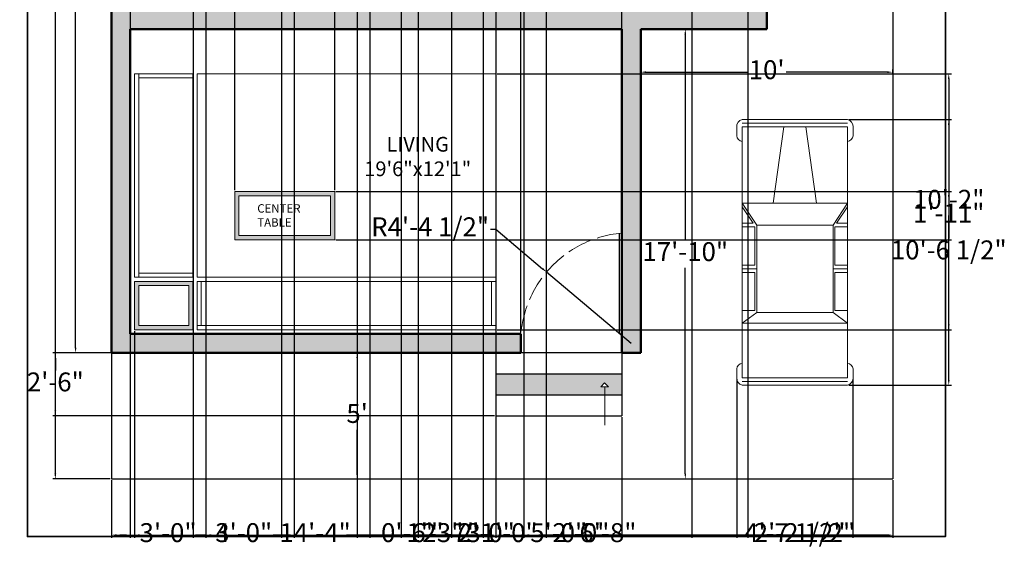
# Model space of a CAD drawing. Units: inches. Extents: x 24899 to 30135, y 37074 to 37745.
# Tile 1 of 3: x 24906 to 25375, y 37074 to 37333. Entities that reach past the tile are written whole.
import ezdxf

# ---------------------------------------------------------------- set-up
doc = ezdxf.new("R2010")
doc.units = ezdxf.units.IN
doc.linetypes.add('ACAD_ISO02W100', pattern=[15, 12, -3])
for name, color, linetype, lineweight in [('A-ANNO-DIMS', 2, 'Continuous', 18), ('A-ANNO-SYMB', 7, 'Continuous', 18), ('A-ANNO-TEXT', 7, 'Continuous', 18), ('A-ANNO-TTLB', 7, 'Continuous', 35), ('A-AREA-IDEN', 7, 'Continuous', 25), ('A-DOOR', 4, 'Continuous', 25), ('A-DOOR-SWNG', 4, 'ACAD_ISO02W100', 13), ('A-EQPM-VEHI', 8, 'Continuous', 13), ('A-FLOR-STRS', 7, 'Continuous', 25), ('A-FLOR-STRS-PATT', 8, 'Continuous', 13), ('A-FURN', 8, 'Continuous', 18), ('A-WALL', 7, 'Continuous', 50), ('C-PROP', 3, 'Continuous', 25)]:
    doc.layers.add(name, color=color, linetype=linetype, lineweight=lineweight)
doc.layers.add('A-FURN-PATT', color=251, linetype='Continuous', lineweight=13, true_color=0x636466)
doc.layers.add('A-WALL-PATT', color=18, linetype='Continuous', lineweight=13, true_color=0x000000)
doc.styles.get("Standard").update_dxf_attribs({"font": 'arial.ttf'})
doc.dimstyles.new('ISO-25', dxfattribs={"dimtxt": 9, "dimasz": 2.5, "dimexe": 1.25, "dimexo": 0.625, "dimgap": 2, "dimtad": 0, "dimtih": 1, "dimtoh": 1, "dimdec": 1, "dimlunit": 4, "dimtxsty": 'Standard', "dimcen": 2.5, "dimadec": 0, "dimazin": 0, "dimtfac": 0.5, "dimtdec": 1, "dimtmove": 0, "dimatfit": 3, "dimfxl": 1, "dimarcsym": 0})

# ---------------------------------------------------------------- blocks, each defined once
blk = doc.blocks.new('*D2')
at = {"layer": 'A-ANNO-DIMS', "color": 0, "lineweight": -2, "transparency": 16777216}
for p, q in [((24948.85, 37582.43), (24931.16, 37582.43)), ((24932.41, 37579.93), (24932.41, 37385.03)), ((24932.41, 37176.93), (24932.41, 37371.83)), ((24948.85, 37174.43), (24931.16, 37174.43))]:
    blk.add_line(p, q, dxfattribs=at)
at = {"layer": 'A-ANNO-DIMS', "color": 0, "transparency": 16777216}
for points in [[(24932, 37579.93), (24932.83, 37579.93), (24932.41, 37582.43)], [(24932, 37176.93), (24932.83, 37176.93), (24932.41, 37174.43)]]:
    blk.add_solid(points, dxfattribs=at)
at = {"layer": 'Defpoints', "color": 0, "transparency": 16777216}
for p in [(24949.48, 37582.43), (24932.41, 37174.43), (24949.48, 37174.43)]:
    blk.add_point(p, dxfattribs=at)
at = {"layer": 'A-ANNO-DIMS', "color": 0, "transparency": 16777216, "insert": (24932.41, 37378.43), "char_height": 9, "attachment_point": 5}
blk.add_mtext("34'", dxfattribs=at)
blk = doc.blocks.new('*D5')
at = {"layer": 'A-ANNO-DIMS', "color": 0, "lineweight": -2, "transparency": 16777216}
for p, q in [((25201.48, 37307.43), (25201.48, 37309.22)), ((25321.48, 37307.43), (25321.48, 37309.22)), ((25203.98, 37307.97), (25252.26, 37307.97)), ((25318.98, 37307.97), (25270.69, 37307.97))]:
    blk.add_line(p, q, dxfattribs=at)
at = {"layer": 'A-ANNO-DIMS', "color": 0, "transparency": 16777216}
for points in [[(25203.98, 37308.38), (25203.98, 37307.55), (25201.48, 37307.97)], [(25318.98, 37308.38), (25318.98, 37307.55), (25321.48, 37307.97)]]:
    blk.add_solid(points, dxfattribs=at)
at = {"layer": 'Defpoints', "color": 0, "transparency": 16777216}
for p in [(25201.48, 37306.81), (25321.48, 37307.97), (25321.48, 37306.81)]:
    blk.add_point(p, dxfattribs=at)
at = {"layer": 'A-ANNO-DIMS', "color": 0, "transparency": 16777216, "insert": (25261.48, 37307.97), "char_height": 9, "attachment_point": 5}
blk.add_mtext("10'", dxfattribs=at)
blk = doc.blocks.new('*D6')
at = {"layer": 'A-ANNO-DIMS', "color": 0, "lineweight": -2, "transparency": 16777216}
for p, q in [((25223.36, 37328.43), (25223.98, 37328.43)), ((25222.73, 37325.93), (25222.73, 37228.03)), ((25222.73, 37116.93), (25222.73, 37214.84)), ((25223.36, 37114.43), (25223.98, 37114.43))]:
    blk.add_line(p, q, dxfattribs=at)
at = {"layer": 'A-ANNO-DIMS', "color": 0, "transparency": 16777216}
for points in [[(25222.32, 37325.93), (25223.15, 37325.93), (25222.73, 37328.43)], [(25222.32, 37116.93), (25223.15, 37116.93), (25222.73, 37114.43)]]:
    blk.add_solid(points, dxfattribs=at)
at = {"layer": 'Defpoints', "color": 0, "transparency": 16777216}
for p in [(25222.73, 37328.43), (25222.73, 37114.43), (25222.73, 37114.43)]:
    blk.add_point(p, dxfattribs=at)
at = {"layer": 'A-ANNO-DIMS', "color": 0, "transparency": 16777216, "insert": (25222.73, 37221.43), "char_height": 9, "attachment_point": 5}
blk.add_mtext('17\'-10"', dxfattribs=at)
blk = doc.blocks.new('*D9')
at = {"layer": 'A-ANNO-DIMS', "color": 0, "lineweight": -2, "transparency": 16777216}
for p, q in [((25067.12, 37174.43), (25067.74, 37174.43)), ((25066.49, 37171.93), (25066.49, 37151.01)), ((25066.49, 37116.93), (25066.49, 37137.86)), ((25067.12, 37114.43), (25067.74, 37114.43))]:
    blk.add_line(p, q, dxfattribs=at)
at = {"layer": 'A-ANNO-DIMS', "color": 0, "transparency": 16777216}
for points in [[(25066.08, 37171.93), (25066.91, 37171.93), (25066.49, 37174.43)], [(25066.08, 37116.93), (25066.91, 37116.93), (25066.49, 37114.43)]]:
    blk.add_solid(points, dxfattribs=at)
at = {"layer": 'Defpoints', "color": 0, "transparency": 16777216}
for p in [(25066.49, 37174.43), (25066.49, 37114.43), (25066.49, 37114.43)]:
    blk.add_point(p, dxfattribs=at)
at = {"layer": 'A-ANNO-DIMS', "color": 0, "transparency": 16777216, "insert": (25066.49, 37144.43), "char_height": 9, "attachment_point": 5}
blk.add_mtext("5'", dxfattribs=at)
blk = doc.blocks.new('*U11')
for p, q in [((0.1, -0.41), (0.1, 38.35)), ((2.77, -0.41), (2.77, 38.31)), ((5.44, 42.31), (12.12, 42.31)), ((5.44, -0.41), (5.44, 38.24)), ((5.45, 38.31), (16.12, 38.31)), ((16.12, 38.31), (180.34, 38.31)), ((61.52, -0.41), (61.52, 38.31)), ((61.52, 38.31), (77.54, 27.62)), ((64.19, 38.31), (76.2, 30.29)), ((76.2, 30.29), (76.2, 38.31)), ((78.87, 38.31), (78.87, 28.96)), ((106.91, 28.96), (106.91, 38.31)), ((109.58, 27.62), (109.58, 38.31)), ((112.25, 38.31), (112.25, 28.96)), ((140.29, 28.96), (140.29, 38.31)), ((141.62, 27.62), (149.64, 38.31)), ((149.64, -0.41), (149.64, 38.31)), ((189.69, 38.31), (179.01, 38.31)), ((189.69, 42.31), (183.01, 42.31)), ((189.69, -0.41), (189.69, 38.24)), ((192.36, -0.41), (192.36, 38.31)), ((195.03, -0.41), (195.03, 38.35)), ((78.87, 28.96), (106.91, 28.96)), ((112.25, 28.96), (140.29, 28.96)), ((77.54, 27.62), (141.62, 27.62)), ((77.54, -0.41), (77.54, 27.62)), ((141.62, -0.41), (141.62, 27.62)), ((5.44, 7.6), (61.52, 15.61)), ((0.1, -0.42), (0.1, -39.18)), ((2.77, -0.41), (2.77, -39.13)), ((5.44, -0.42), (5.44, -39.07)), ((61.52, -0.41), (61.52, -39.13)), ((77.54, -0.41), (77.54, -28.45)), ((141.62, -0.41), (141.62, -28.45)), ((149.64, -0.41), (149.64, -39.13)), ((189.69, -0.42), (189.69, -39.07)), ((192.36, -0.41), (192.36, -39.13)), ((195.03, -0.42), (195.03, -39.18)), ((5.44, -8.42), (61.52, -16.43)), ((61.52, -39.13), (77.54, -28.45)), ((77.54, -28.45), (141.62, -28.45)), ((109.58, -28.45), (109.58, -39.13)), ((141.62, -28.45), (149.64, -39.13)), ((64.19, -39.13), (76.2, -31.12)), ((76.2, -31.12), (76.2, -39.13)), ((78.87, -39.13), (78.87, -29.79)), ((78.87, -29.79), (106.91, -29.79)), ((106.91, -29.79), (106.91, -39.13)), ((112.25, -29.79), (140.29, -29.79)), ((112.25, -39.13), (112.25, -29.79)), ((140.29, -29.79), (140.29, -39.13)), ((5.44, -43.14), (12.12, -43.14)), ((5.45, -39.13), (16.12, -39.13)), ((16.12, -39.13), (180.34, -39.13)), ((189.69, -39.13), (179.01, -39.13)), ((189.69, -43.14), (183.01, -43.14))]:
    blk.add_line(p, q)
for centre, radius, start, end in [((5.06, 37.26), 5.06, 85.64554, 168.0943), ((11.45, 37.64), 4.72, 8.13011, 81.86996), ((183.68, 37.64), 4.72, 98.13004, 171.8699), ((190.07, 37.26), 5.06, 11.90574, 94.35446), ((5.06, -38.09), 5.06, 191.9057, 274.3545), ((11.45, -38.46), 4.72, 278.13, 351.8699), ((183.68, -38.46), 4.72, 188.1301, 261.87), ((190.07, -38.09), 5.06, 265.6455, 348.0943)]:
    blk.add_arc(centre, radius, start, end)
blk = doc.blocks.new('*D17')
at = {"layer": 'A-ANNO-DIMS', "color": 0, "lineweight": -2, "transparency": 16777216}
for p, q in [((24949.48, 37113.81), (24949.48, 37086.48)), ((25321.48, 37113.81), (25321.48, 37086.48)), ((24951.98, 37087.73), (25118.02, 37087.73)), ((25318.98, 37087.73), (25152.93, 37087.73))]:
    blk.add_line(p, q, dxfattribs=at)
at = {"layer": 'A-ANNO-DIMS', "color": 0, "transparency": 16777216}
for points in [[(24951.98, 37088.15), (24951.98, 37087.32), (24949.48, 37087.73)], [(25318.98, 37088.15), (25318.98, 37087.32), (25321.48, 37087.73)]]:
    blk.add_solid(points, dxfattribs=at)
at = {"layer": 'Defpoints', "color": 0, "transparency": 16777216}
for p in [(24949.48, 37114.43), (25321.48, 37114.43), (25321.48, 37087.73)]:
    blk.add_point(p, dxfattribs=at)
at = {"layer": 'A-ANNO-DIMS', "color": 0, "transparency": 16777216, "insert": (25135.48, 37087.73), "char_height": 9, "attachment_point": 5}
blk.add_mtext('31\'-0"', dxfattribs=at)
blk = doc.blocks.new('*D18')
at = {"layer": 'A-ANNO-DIMS', "color": 0, "lineweight": -2, "transparency": 16777216}
for p, q in [((24948.85, 37630.43), (24921.53, 37630.43)), ((24922.78, 37627.93), (24922.78, 37379.03)), ((24922.78, 37116.93), (24922.78, 37365.83)), ((24948.85, 37114.43), (24921.53, 37114.43))]:
    blk.add_line(p, q, dxfattribs=at)
at = {"layer": 'A-ANNO-DIMS', "color": 0, "transparency": 16777216}
for points in [[(24922.36, 37627.93), (24923.19, 37627.93), (24922.78, 37630.43)], [(24922.36, 37116.93), (24923.19, 37116.93), (24922.78, 37114.43)]]:
    blk.add_solid(points, dxfattribs=at)
at = {"layer": 'Defpoints', "color": 0, "transparency": 16777216}
for p in [(24949.48, 37630.43), (24922.78, 37114.43), (24949.48, 37114.43)]:
    blk.add_point(p, dxfattribs=at)
at = {"layer": 'A-ANNO-DIMS', "color": 0, "transparency": 16777216, "insert": (24922.78, 37372.43), "char_height": 9, "attachment_point": 5}
blk.add_mtext('43\'-0"', dxfattribs=at)
blk = doc.blocks.new('*D19')
at = {"layer": 'A-ANNO-DIMS', "color": 0, "lineweight": -2, "transparency": 16777216}
for p, q in [((24958.48, 37572.81), (24958.48, 37086.48)), ((24994.48, 37572.81), (24994.48, 37086.48)), ((24955.98, 37087.73), (24953.48, 37087.73)), ((24958.48, 37087.73), (24962.52, 37087.73)), ((24994.48, 37087.73), (24990.44, 37087.73)), ((24996.98, 37087.73), (24999.48, 37087.73))]:
    blk.add_line(p, q, dxfattribs=at)
at = {"layer": 'A-ANNO-DIMS', "color": 0, "transparency": 16777216}
for points in [[(24955.98, 37088.15), (24955.98, 37087.32), (24958.48, 37087.73)], [(24996.98, 37088.15), (24996.98, 37087.32), (24994.48, 37087.73)]]:
    blk.add_solid(points, dxfattribs=at)
at = {"layer": 'Defpoints', "color": 0, "transparency": 16777216}
for p in [(24958.48, 37573.43), (24994.48, 37573.43), (24994.48, 37087.73)]:
    blk.add_point(p, dxfattribs=at)
at = {"layer": 'A-ANNO-DIMS', "color": 0, "transparency": 16777216, "insert": (24976.48, 37087.73), "char_height": 9, "attachment_point": 5}
blk.add_mtext('3\'-0"', dxfattribs=at)
blk = doc.blocks.new('*D20')
at = {"layer": 'A-ANNO-DIMS', "color": 0, "lineweight": -2, "transparency": 16777216}
for p, q in [((24994.48, 37572.81), (24994.48, 37086.48)), ((25030.48, 37572.81), (25030.48, 37086.48)), ((24991.98, 37087.73), (24989.48, 37087.73)), ((24994.48, 37087.73), (24998.52, 37087.73)), ((25030.48, 37087.73), (25026.44, 37087.73)), ((25032.98, 37087.73), (25035.48, 37087.73))]:
    blk.add_line(p, q, dxfattribs=at)
at = {"layer": 'A-ANNO-DIMS', "color": 0, "transparency": 16777216}
for points in [[(24991.98, 37088.15), (24991.98, 37087.32), (24994.48, 37087.73)], [(25032.98, 37088.15), (25032.98, 37087.32), (25030.48, 37087.73)]]:
    blk.add_solid(points, dxfattribs=at)
at = {"layer": 'Defpoints', "color": 0, "transparency": 16777216}
for p in [(24994.48, 37573.43), (25030.48, 37573.43), (25030.48, 37087.73)]:
    blk.add_point(p, dxfattribs=at)
at = {"layer": 'A-ANNO-DIMS', "color": 0, "transparency": 16777216, "insert": (25012.48, 37087.73), "char_height": 9, "attachment_point": 5}
blk.add_mtext('3\'-0"', dxfattribs=at)
blk = doc.blocks.new('*D21')
at = {"layer": 'A-ANNO-DIMS', "color": 0, "lineweight": -2, "transparency": 16777216}
for p, q in [((25072.48, 37572.81), (25072.48, 37086.48)), ((25087.48, 37572.81), (25087.48, 37086.48)), ((25074.98, 37087.73), (25084.98, 37087.73)), ((25087.48, 37087.73), (25089.98, 37087.73))]:
    blk.add_line(p, q, dxfattribs=at)
at = {"layer": 'A-ANNO-DIMS', "color": 0, "transparency": 16777216}
for points in [[(25074.98, 37088.15), (25074.98, 37087.32), (25072.48, 37087.73)], [(25084.98, 37088.15), (25084.98, 37087.32), (25087.48, 37087.73)]]:
    blk.add_solid(points, dxfattribs=at)
at = {"layer": 'Defpoints', "color": 0, "transparency": 16777216}
for p in [(25072.48, 37573.43), (25087.48, 37573.43), (25087.48, 37087.73)]:
    blk.add_point(p, dxfattribs=at)
at = {"layer": 'A-ANNO-DIMS', "color": 0, "transparency": 16777216, "insert": (25103.52, 37087.73), "char_height": 9, "attachment_point": 5}
blk.add_mtext('1\'-3"', dxfattribs=at)
blk = doc.blocks.new('*D22')
at = {"layer": 'A-ANNO-DIMS', "color": 0, "lineweight": -2, "transparency": 16777216}
for p, q in [((25087.48, 37572.81), (25087.48, 37086.48)), ((25111.48, 37572.81), (25111.48, 37086.48)), ((25089.98, 37087.73), (25108.98, 37087.73)), ((25111.48, 37087.73), (25113.98, 37087.73))]:
    blk.add_line(p, q, dxfattribs=at)
at = {"layer": 'A-ANNO-DIMS', "color": 0, "transparency": 16777216}
for points in [[(25089.98, 37088.15), (25089.98, 37087.32), (25087.48, 37087.73)], [(25108.98, 37088.15), (25108.98, 37087.32), (25111.48, 37087.73)]]:
    blk.add_solid(points, dxfattribs=at)
at = {"layer": 'Defpoints', "color": 0, "transparency": 16777216}
for p in [(25087.48, 37573.43), (25111.48, 37573.43), (25111.48, 37087.73)]:
    blk.add_point(p, dxfattribs=at)
at = {"layer": 'A-ANNO-DIMS', "color": 0, "transparency": 16777216, "insert": (25128.02, 37087.73), "char_height": 9, "attachment_point": 5}
blk.add_mtext('2\'-0"', dxfattribs=at)
blk = doc.blocks.new('*D23')
at = {"layer": 'A-ANNO-DIMS', "color": 0, "lineweight": -2, "transparency": 16777216}
for p, q in [((25132.48, 37572.81), (25132.48, 37086.48)), ((25156.48, 37572.81), (25156.48, 37086.48)), ((25134.98, 37087.73), (25153.98, 37087.73)), ((25156.48, 37087.73), (25158.98, 37087.73))]:
    blk.add_line(p, q, dxfattribs=at)
at = {"layer": 'A-ANNO-DIMS', "color": 0, "transparency": 16777216}
for points in [[(25134.98, 37088.15), (25134.98, 37087.32), (25132.48, 37087.73)], [(25153.98, 37088.15), (25153.98, 37087.32), (25156.48, 37087.73)]]:
    blk.add_solid(points, dxfattribs=at)
at = {"layer": 'Defpoints', "color": 0, "transparency": 16777216}
for p in [(25132.48, 37573.43), (25156.48, 37573.43), (25156.48, 37087.73)]:
    blk.add_point(p, dxfattribs=at)
at = {"layer": 'A-ANNO-DIMS', "color": 0, "transparency": 16777216, "insert": (25173.02, 37087.73), "char_height": 9, "attachment_point": 5}
blk.add_mtext('2\'-0"', dxfattribs=at)
blk = doc.blocks.new('*D26')
at = {"layer": 'A-ANNO-DIMS', "color": 0, "lineweight": -2, "transparency": 16777216}
for p, q in [((24988.48, 37464.81), (24988.48, 37086.48)), ((25036.48, 37464.81), (25036.48, 37086.48)), ((24990.98, 37087.73), (24998.33, 37087.73)), ((25033.98, 37087.73), (25026.62, 37087.73))]:
    blk.add_line(p, q, dxfattribs=at)
at = {"layer": 'A-ANNO-DIMS', "color": 0, "transparency": 16777216}
for points in [[(24990.98, 37088.15), (24990.98, 37087.32), (24988.48, 37087.73)], [(25033.98, 37088.15), (25033.98, 37087.32), (25036.48, 37087.73)]]:
    blk.add_solid(points, dxfattribs=at)
at = {"layer": 'Defpoints', "color": 0, "transparency": 16777216}
for p in [(24988.48, 37465.43), (25036.48, 37465.43), (25036.48, 37087.73)]:
    blk.add_point(p, dxfattribs=at)
at = {"layer": 'A-ANNO-DIMS', "color": 0, "transparency": 16777216, "insert": (25012.48, 37087.73), "char_height": 9, "attachment_point": 5}
blk.add_mtext('4\'-0"', dxfattribs=at)
blk = doc.blocks.new('*D27')
at = {"layer": 'A-ANNO-DIMS', "color": 0, "lineweight": -2, "transparency": 16777216}
for p, q in [((25095.48, 37470.81), (25095.48, 37086.48)), ((25126.48, 37470.81), (25126.48, 37086.48)), ((25092.98, 37087.73), (25090.48, 37087.73)), ((25095.48, 37087.73), (25096.94, 37087.73)), ((25126.48, 37087.73), (25125.02, 37087.73)), ((25128.98, 37087.73), (25131.48, 37087.73))]:
    blk.add_line(p, q, dxfattribs=at)
at = {"layer": 'A-ANNO-DIMS', "color": 0, "transparency": 16777216}
for points in [[(25092.98, 37088.15), (25092.98, 37087.32), (25095.48, 37087.73)], [(25128.98, 37088.15), (25128.98, 37087.32), (25126.48, 37087.73)]]:
    blk.add_solid(points, dxfattribs=at)
at = {"layer": 'Defpoints', "color": 0, "transparency": 16777216}
for p in [(25095.48, 37471.43), (25126.48, 37471.43), (25126.48, 37087.73)]:
    blk.add_point(p, dxfattribs=at)
at = {"layer": 'A-ANNO-DIMS', "color": 0, "transparency": 16777216, "insert": (25110.98, 37087.73), "char_height": 9, "attachment_point": 5}
blk.add_mtext('2\'-7"', dxfattribs=at)
blk = doc.blocks.new('*D30')
at = {"layer": 'A-ANNO-DIMS', "color": 0, "lineweight": -2, "transparency": 16777216}
for p, q in [((25145.9, 37336.81), (25145.9, 37086.48)), ((25225.9, 37336.81), (25225.9, 37086.48)), ((25148.4, 37087.73), (25171.91, 37087.73)), ((25223.4, 37087.73), (25199.89, 37087.73))]:
    blk.add_line(p, q, dxfattribs=at)
at = {"layer": 'A-ANNO-DIMS', "color": 0, "transparency": 16777216}
for points in [[(25148.4, 37088.15), (25148.4, 37087.32), (25145.9, 37087.73)], [(25223.4, 37088.15), (25223.4, 37087.32), (25225.9, 37087.73)]]:
    blk.add_solid(points, dxfattribs=at)
at = {"layer": 'Defpoints', "color": 0, "transparency": 16777216}
for p in [(25145.9, 37337.43), (25225.9, 37337.43), (25225.9, 37087.73)]:
    blk.add_point(p, dxfattribs=at)
at = {"layer": 'A-ANNO-DIMS', "color": 0, "transparency": 16777216, "insert": (25185.9, 37087.73), "char_height": 9, "attachment_point": 5}
blk.add_mtext('6\'-8"', dxfattribs=at)
blk = doc.blocks.new('*D31')
at = {"layer": 'A-ANNO-DIMS', "color": 0, "lineweight": -2, "transparency": 16777216}
for p, q in [((25225.9, 37336.81), (25225.9, 37086.48)), ((25252.48, 37336.81), (25252.48, 37086.48)), ((25228.4, 37087.73), (25249.98, 37087.73)), ((25252.48, 37087.73), (25254.98, 37087.73))]:
    blk.add_line(p, q, dxfattribs=at)
at = {"layer": 'A-ANNO-DIMS', "color": 0, "transparency": 16777216}
for points in [[(25228.4, 37088.15), (25228.4, 37087.32), (25225.9, 37087.73)], [(25249.98, 37088.15), (25249.98, 37087.32), (25252.48, 37087.73)]]:
    blk.add_solid(points, dxfattribs=at)
at = {"layer": 'Defpoints', "color": 0, "transparency": 16777216}
for p in [(25225.9, 37337.43), (25252.48, 37337.43), (25252.48, 37087.73)]:
    blk.add_point(p, dxfattribs=at)
at = {"layer": 'A-ANNO-DIMS', "color": 0, "transparency": 16777216, "insert": (25279.5, 37087.73), "char_height": 9, "attachment_point": 5}
blk.add_mtext('2\'-2 1/2"', dxfattribs=at)
blk = doc.blocks.new('*D33')
at = {"layer": 'A-ANNO-DIMS', "color": 0, "lineweight": -2, "transparency": 16777216}
for p, q in [((25144.48, 37184.06), (25144.48, 37658.38)), ((25146.98, 37657.13), (25154.33, 37657.13)), ((25189.98, 37657.13), (25182.62, 37657.13)), ((25192.48, 37184.06), (25192.48, 37658.38))]:
    blk.add_line(p, q, dxfattribs=at)
at = {"layer": 'A-ANNO-DIMS', "color": 0, "transparency": 16777216}
for points in [[(25146.98, 37657.55), (25146.98, 37656.72), (25144.48, 37657.13)], [(25189.98, 37657.55), (25189.98, 37656.72), (25192.48, 37657.13)]]:
    blk.add_solid(points, dxfattribs=at)
at = {"layer": 'Defpoints', "color": 0, "transparency": 16777216}
for p in [(25192.48, 37657.13), (25144.48, 37183.43), (25192.48, 37183.43)]:
    blk.add_point(p, dxfattribs=at)
at = {"layer": 'A-ANNO-DIMS', "color": 0, "transparency": 16777216, "insert": (25168.48, 37657.13), "char_height": 9, "attachment_point": 5}
blk.add_mtext('4\'-0"', dxfattribs=at)
blk = doc.blocks.new('*D34')
at = {"layer": 'A-ANNO-DIMS', "color": 0, "lineweight": -2, "transparency": 16777216}
for p, q in [((25132.48, 37143.81), (25132.48, 37086.48)), ((25192.48, 37143.81), (25192.48, 37086.48)), ((25134.98, 37087.73), (25148.51, 37087.73)), ((25189.98, 37087.73), (25176.44, 37087.73))]:
    blk.add_line(p, q, dxfattribs=at)
at = {"layer": 'A-ANNO-DIMS', "color": 0, "transparency": 16777216}
for points in [[(25134.98, 37088.15), (25134.98, 37087.32), (25132.48, 37087.73)], [(25189.98, 37088.15), (25189.98, 37087.32), (25192.48, 37087.73)]]:
    blk.add_solid(points, dxfattribs=at)
at = {"layer": 'Defpoints', "color": 0, "transparency": 16777216}
for p in [(25132.48, 37144.43), (25192.48, 37144.43), (25192.48, 37087.73)]:
    blk.add_point(p, dxfattribs=at)
at = {"layer": 'A-ANNO-DIMS', "color": 0, "transparency": 16777216, "insert": (25162.48, 37087.73), "char_height": 9, "attachment_point": 5}
blk.add_mtext('5\'-0"', dxfattribs=at)
blk = doc.blocks.new('*D35')
at = {"layer": 'A-ANNO-DIMS', "color": 0, "lineweight": -2, "transparency": 16777216}
for p, q in [((25131.85, 37174.43), (24921.53, 37174.43)), ((24922.78, 37171.93), (24922.78, 37166.03)), ((24922.78, 37146.93), (24922.78, 37152.84)), ((25131.85, 37144.43), (24921.53, 37144.43))]:
    blk.add_line(p, q, dxfattribs=at)
at = {"layer": 'A-ANNO-DIMS', "color": 0, "transparency": 16777216}
for points in [[(24922.36, 37171.93), (24923.19, 37171.93), (24922.78, 37174.43)], [(24922.36, 37146.93), (24923.19, 37146.93), (24922.78, 37144.43)]]:
    blk.add_solid(points, dxfattribs=at)
at = {"layer": 'Defpoints', "color": 0, "transparency": 16777216}
for p in [(24922.78, 37174.43), (25132.48, 37174.43), (25132.48, 37144.43)]:
    blk.add_point(p, dxfattribs=at)
at = {"layer": 'A-ANNO-DIMS', "color": 0, "transparency": 16777216, "insert": (24922.78, 37159.43), "char_height": 9, "attachment_point": 5}
blk.add_mtext('2\'-6"', dxfattribs=at)
blk = doc.blocks.new('*D36')
at = {"layer": 'A-ANNO-DIMS', "color": 0, "lineweight": -2, "transparency": 16777216}
for p, q in [((25008.22, 37251.81), (25008.22, 37658.38)), ((25010.72, 37657.13), (25053.29, 37657.13)), ((25055.79, 37251.81), (25055.79, 37658.38)), ((25055.79, 37657.13), (25058.29, 37657.13))]:
    blk.add_line(p, q, dxfattribs=at)
at = {"layer": 'A-ANNO-DIMS', "color": 0, "transparency": 16777216}
for points in [[(25010.72, 37657.55), (25010.72, 37656.72), (25008.22, 37657.13)], [(25053.29, 37657.55), (25053.29, 37656.72), (25055.79, 37657.13)]]:
    blk.add_solid(points, dxfattribs=at)
at = {"layer": 'Defpoints', "color": 0, "transparency": 16777216}
for p in [(25055.79, 37657.13), (25008.22, 37251.19), (25055.79, 37251.19)]:
    blk.add_point(p, dxfattribs=at)
at = {"layer": 'A-ANNO-DIMS', "color": 0, "transparency": 16777216, "insert": (25086.23, 37657.13), "char_height": 9, "attachment_point": 5}
blk.add_mtext('3\'-11 1/2"', dxfattribs=at)
blk = doc.blocks.new('*D37')
at = {"layer": 'A-ANNO-DIMS', "color": 0, "lineweight": -2, "transparency": 16777216}
for p, q in [((25056.41, 37251.19), (25349.43, 37251.19)), ((25348.18, 37248.69), (25348.18, 37246.25)), ((25348.18, 37230.78), (25348.18, 37233.22)), ((25056.41, 37228.28), (25349.43, 37228.28))]:
    blk.add_line(p, q, dxfattribs=at)
at = {"layer": 'A-ANNO-DIMS', "color": 0, "transparency": 16777216}
for points in [[(25347.76, 37248.69), (25348.59, 37248.69), (25348.18, 37251.19)], [(25347.76, 37230.78), (25348.59, 37230.78), (25348.18, 37228.28)]]:
    blk.add_solid(points, dxfattribs=at)
at = {"layer": 'Defpoints', "color": 0, "transparency": 16777216}
for p in [(25055.79, 37251.19), (25348.18, 37251.19), (25055.79, 37228.28)]:
    blk.add_point(p, dxfattribs=at)
at = {"layer": 'A-ANNO-DIMS', "color": 0, "transparency": 16777216, "insert": (25348.18, 37239.74), "char_height": 9, "attachment_point": 5}
blk.add_mtext('1\'-11"', dxfattribs=at)
blk = doc.blocks.new('*D38')
at = {"layer": 'A-ANNO-DIMS', "color": 0, "lineweight": -2, "transparency": 16777216}
for p, q in [((24960.48, 37184.81), (24960.48, 37086.48)), ((25132.48, 37184.81), (25132.48, 37086.48)), ((24962.98, 37087.73), (25029.44, 37087.73)), ((25129.98, 37087.73), (25063.51, 37087.73))]:
    blk.add_line(p, q, dxfattribs=at)
at = {"layer": 'A-ANNO-DIMS', "color": 0, "transparency": 16777216}
for points in [[(24962.98, 37088.15), (24962.98, 37087.32), (24960.48, 37087.73)], [(25129.98, 37088.15), (25129.98, 37087.32), (25132.48, 37087.73)]]:
    blk.add_solid(points, dxfattribs=at)
at = {"layer": 'Defpoints', "color": 0, "transparency": 16777216}
for p in [(24960.48, 37185.43), (25132.48, 37185.43), (25132.48, 37087.73)]:
    blk.add_point(p, dxfattribs=at)
at = {"layer": 'A-ANNO-DIMS', "color": 0, "transparency": 16777216, "insert": (25046.48, 37087.73), "char_height": 9, "attachment_point": 5}
blk.add_mtext('14\'-4"', dxfattribs=at)
blk = doc.blocks.new('*D39')
at = {"layer": 'A-ANNO-DIMS', "color": 0, "lineweight": -2, "transparency": 16777216}
for p, q in [((25133.1, 37307.2), (25349.43, 37307.2)), ((25348.18, 37304.7), (25348.18, 37252.91)), ((25348.18, 37187.93), (25348.18, 37239.72)), ((25133.1, 37185.43), (25349.43, 37185.43))]:
    blk.add_line(p, q, dxfattribs=at)
at = {"layer": 'A-ANNO-DIMS', "color": 0, "transparency": 16777216}
for points in [[(25347.76, 37304.7), (25348.59, 37304.7), (25348.18, 37307.2)], [(25347.76, 37187.93), (25348.59, 37187.93), (25348.18, 37185.43)]]:
    blk.add_solid(points, dxfattribs=at)
at = {"layer": 'Defpoints', "color": 0, "transparency": 16777216}
for p in [(25132.48, 37307.2), (25348.18, 37307.2), (25132.48, 37185.43)]:
    blk.add_point(p, dxfattribs=at)
at = {"layer": 'A-ANNO-DIMS', "color": 0, "transparency": 16777216, "insert": (25348.18, 37246.32), "char_height": 9, "attachment_point": 5}
blk.add_mtext('10\'-2"', dxfattribs=at)
blk = doc.blocks.new('*D40')
at = {"layer": 'A-ANNO-DIMS', "color": 0, "lineweight": -2, "transparency": 16777216}
for p, q in [((25247.19, 37161.89), (25247.19, 37086.48)), ((25302.58, 37161.89), (25302.58, 37086.48)), ((25244.69, 37087.73), (25242.19, 37087.73)), ((25247.19, 37087.73), (25250.26, 37087.73)), ((25302.58, 37087.73), (25299.52, 37087.73)), ((25305.08, 37087.73), (25307.58, 37087.73))]:
    blk.add_line(p, q, dxfattribs=at)
at = {"layer": 'A-ANNO-DIMS', "color": 0, "transparency": 16777216}
for points in [[(25244.69, 37088.15), (25244.69, 37087.32), (25247.19, 37087.73)], [(25305.08, 37088.15), (25305.08, 37087.32), (25302.58, 37087.73)]]:
    blk.add_solid(points, dxfattribs=at)
at = {"layer": 'Defpoints', "color": 0, "transparency": 16777216}
for p in [(25247.19, 37162.52), (25302.58, 37162.52), (25302.58, 37087.73)]:
    blk.add_point(p, dxfattribs=at)
at = {"layer": 'A-ANNO-DIMS', "color": 0, "transparency": 16777216, "insert": (25274.89, 37087.73), "char_height": 9, "attachment_point": 5}
blk.add_mtext('4\'-7 1/2"', dxfattribs=at)
blk = doc.blocks.new('*D41')
at = {"layer": 'A-ANNO-DIMS', "color": 0, "lineweight": -2, "transparency": 16777216}
for p, q in [((25300.61, 37285.41), (25349.43, 37285.41)), ((25348.18, 37282.91), (25348.18, 37228.89)), ((25348.18, 37161.56), (25348.18, 37215.58)), ((25300.61, 37159.06), (25349.43, 37159.06))]:
    blk.add_line(p, q, dxfattribs=at)
at = {"layer": 'A-ANNO-DIMS', "color": 0, "transparency": 16777216}
for points in [[(25347.76, 37282.91), (25348.59, 37282.91), (25348.18, 37285.41)], [(25347.76, 37161.56), (25348.59, 37161.56), (25348.18, 37159.06)]]:
    blk.add_solid(points, dxfattribs=at)
at = {"layer": 'Defpoints', "color": 0, "transparency": 16777216}
for p in [(25299.99, 37285.41), (25348.18, 37285.41), (25299.99, 37159.06)]:
    blk.add_point(p, dxfattribs=at)
at = {"layer": 'A-ANNO-DIMS', "color": 0, "transparency": 16777216, "insert": (25348.18, 37222.24), "char_height": 9, "attachment_point": 5}
blk.add_mtext('10\'-6 1/2"', dxfattribs=at)
blk = doc.blocks.new('*D45')
at = {"layer": 'A-ANNO-DIMS', "color": 0, "lineweight": -2, "transparency": 16777216}
for p, q in [((25072.48, 37470.81), (25072.48, 37086.48)), ((25066.48, 37464.81), (25066.48, 37086.48)), ((25063.98, 37087.73), (25061.48, 37087.73)), ((25066.48, 37087.73), (25072.48, 37087.73)), ((25074.98, 37087.73), (25077.48, 37087.73))]:
    blk.add_line(p, q, dxfattribs=at)
at = {"layer": 'A-ANNO-DIMS', "color": 0, "transparency": 16777216}
for points in [[(25063.98, 37088.15), (25063.98, 37087.32), (25066.48, 37087.73)], [(25074.98, 37088.15), (25074.98, 37087.32), (25072.48, 37087.73)]]:
    blk.add_solid(points, dxfattribs=at)
at = {"layer": 'Defpoints', "color": 0, "transparency": 16777216}
for p in [(25072.48, 37471.43), (25066.48, 37465.43), (25072.48, 37087.73)]:
    blk.add_point(p, dxfattribs=at)
at = {"layer": 'A-ANNO-DIMS', "color": 0, "transparency": 16777216, "insert": (25091.44, 37087.73), "char_height": 9, "attachment_point": 5}
blk.add_mtext('0\'-6"', dxfattribs=at)
blk = doc.blocks.new('*D46')
at = {"layer": 'A-ANNO-DIMS', "color": 0, "lineweight": -2, "transparency": 16777216}
for p, q in [((25129.99, 37233.24), (25132.49, 37233.24)), ((25132.49, 37233.24), (25154.76, 37214.48)), ((25196.98, 37178.93), (25156.67, 37212.87))]:
    blk.add_line(p, q, dxfattribs=at)
at = {"layer": 'A-ANNO-DIMS', "color": 0, "transparency": 16777216}
blk.add_solid([(25155.03, 37214.8), (25154.49, 37214.17), (25156.67, 37212.87)], dxfattribs=at)
at = {"layer": 'Defpoints', "color": 0, "transparency": 16777216}
for p in [(25156.67, 37212.87), (25196.98, 37178.93)]:
    blk.add_point(p, dxfattribs=at)
at = {"layer": 'A-ANNO-DIMS', "color": 0, "transparency": 16777216, "insert": (25101.23, 37233.24), "char_height": 9, "attachment_point": 5}
blk.add_mtext('R4\'-4 1/2"', dxfattribs=at)

msp = doc.modelspace()

# ---------------------------------------------------------------- hatches: boundary and pattern name
at = {"layer": 'A-FLOR-STRS-PATT'}
h = msp.add_hatch(color=256, dxfattribs=at)
h.dxf.hatch_style = 1
h.paths.add_polyline_path([(25192.48, 37164.43), (25132.48, 37164.43), (25132.48, 37154.43), (25184.38, 37154.43), (25184.38, 37158.3), (25182.5, 37158.3), (25184.32, 37160.13), (25186.18, 37158.28), (25184.38, 37158.28), (25184.38, 37154.43), (25192.48, 37154.43)])
at = {"layer": 'A-FURN-PATT'}
h = msp.add_hatch(color=256, dxfattribs=at)
h.dxf.hatch_style = 1
h.paths.add_polyline_path([(25055.79, 37251.19), (25008.22, 37251.19), (25008.22, 37228.28), (25055.79, 37228.28)])
h.paths.add_polyline_path([(25010.22, 37249.19), (25053.79, 37249.19), (25053.79, 37230.28), (25010.22, 37230.28)], flags=16)
h.paths.add_polyline_path([(24988.27, 37208.4), (24960.48, 37208.4), (24960.48, 37185.43), (24988.27, 37185.43)])
h.paths.add_polyline_path([(24986.27, 37187.43), (24962.48, 37187.43), (24962.48, 37206.4), (24986.27, 37206.4)], flags=16)
at = {"layer": 'A-WALL-PATT'}
h = msp.add_hatch(color=256, dxfattribs=at)
h.dxf.hatch_style = 1
h.paths.add_polyline_path([(25261.48, 37582.43), (25228.48, 37582.43), (25228.48, 37573.43), (25252.48, 37573.43), (25252.48, 37405.43), (25169.48, 37405.43, -0.038405), (25169.48, 37399.43), (25252.48, 37399.43), (25252.48, 37337.43), (25201.48, 37337.43), (24958.48, 37337.43), (24958.48, 37465.43), (24988.48, 37465.43), (24988.48, 37471.43), (24958.48, 37471.43), (24958.48, 37573.43), (24994.48, 37573.43), (24994.48, 37582.43), (24949.48, 37582.43), (24949.48, 37174.43), (25144.48, 37174.43, -0.042779), (25144.48, 37183.43), (24958.48, 37183.43), (24958.48, 37328.43), (25192.48, 37328.43), (25192.48, 37183.43), (25192.48, 37174.43), (25201.48, 37174.43), (25201.48, 37183.43), (25201.48, 37328.43), (25261.48, 37328.43)])
h.paths.add_polyline_path([(25087.48, 37582.43), (25030.48, 37582.43, -0.077125), (25030.48, 37573.43), (25066.48, 37573.43), (25066.48, 37471.43), (25036.48, 37471.43), (25036.48, 37465.43), (25066.48, 37465.43), (25066.48, 37430.04), (25095.6, 37430.04), (25095.6, 37435.01), (25072.48, 37435.01), (25072.48, 37465.43), (25072.48, 37471.43), (25095.48, 37471.43, -0.045361), (25095.48, 37477.43), (25072.48, 37477.43), (25072.48, 37573.43), (25087.48, 37573.43)], flags=0)
h.paths.add_polyline_path([(25156.48, 37582.43), (25111.48, 37582.43), (25111.48, 37573.43), (25126.48, 37573.43), (25126.48, 37477.43), (25126.48, 37471.43), (25126.48, 37399.43), (25132.48, 37399.43), (25132.48, 37405.43), (25132.48, 37471.43), (25132.48, 37573.43), (25156.48, 37573.43)], flags=17)

# ---------------------------------------------------------------- linework, layer by layer
at = {"layer": 'A-ANNO-SYMB'}
for p, q in [((25182.5, 37158.3), (25184.32, 37160.13)), ((25184.32, 37160.13), (25186.18, 37158.28)), ((25184.38, 37158.3), (25182.5, 37158.3)), ((25184.38, 37140.05), (25184.38, 37158.3)), ((25186.18, 37158.28), (25184.38, 37158.28))]:
    msp.add_line(p, q, dxfattribs=at)
at = {"layer": 'A-ANNO-TTLB'}
msp.add_lwpolyline([(24909.5, 37655.83), (25346.61, 37655.83), (25346.61, 37086.99), (24909.5, 37086.99)], close=True, dxfattribs=at)
at = {"layer": 'A-DOOR'}
for p, q in [((25191.48, 37183.43), (25191.48, 37231.43)), ((25192.48, 37183.43), (25192.48, 37231.43)), ((25191.48, 37183.43), (25192.48, 37183.43))]:
    msp.add_line(p, q, dxfattribs=at)
at = {"layer": 'A-DOOR-SWNG'}
msp.add_arc((25196.98, 37178.93), 52.69, 94.8991, 184.8991, dxfattribs=at)
at = {"layer": 'A-FLOR-STRS'}
for p, q in [((25192.48, 37174.43), (25132.48, 37174.43)), ((25132.48, 37174.43), (25132.48, 37144.43)), ((25192.48, 37174.43), (25192.48, 37144.43)), ((25132.48, 37164.43), (25192.48, 37164.43)), ((25132.48, 37154.43), (25192.48, 37154.43)), ((25132.48, 37144.43), (25192.48, 37144.43))]:
    msp.add_line(p, q, dxfattribs=at)
at = {"layer": 'A-FURN'}
for p, q in [((24960.48, 37307.2), (24960.48, 37210.4)), ((24988.27, 37307.2), (24960.48, 37307.2)), ((24962.48, 37307.2), (24962.48, 37210.4)), ((24988.27, 37305.2), (24962.48, 37305.2)), ((24988.27, 37307.2), (24988.27, 37210.4)), ((25132.48, 37307.2), (24990.27, 37307.2)), ((24990.27, 37307.2), (24990.27, 37210.4)), ((25132.48, 37210.4), (25132.48, 37307.2)), ((24988.27, 37210.4), (24960.48, 37210.4)), ((24988.27, 37212.4), (24962.48, 37212.4)), ((24990.27, 37210.4), (25132.48, 37210.4)), ((24960.48, 37208.4), (24960.48, 37185.43)), ((24988.27, 37208.4), (24960.48, 37208.4)), ((24988.27, 37208.4), (24988.27, 37185.43)), ((24990.27, 37208.4), (25132.48, 37208.4)), ((24990.27, 37208.4), (24990.27, 37185.43)), ((24992.27, 37208.4), (24992.27, 37187.43)), ((25130.48, 37208.4), (25130.48, 37187.43)), ((25132.48, 37208.4), (25132.48, 37185.43)), ((24990.27, 37187.43), (25132.48, 37187.43)), ((24988.27, 37185.43), (24960.48, 37185.43)), ((24990.27, 37185.43), (25132.48, 37185.43))]:
    msp.add_line(p, q, dxfattribs=at)
for points in [[(25008.22, 37251.19), (25055.79, 37251.19), (25055.79, 37228.28), (25008.22, 37228.28)], [(25010.22, 37249.19), (25053.79, 37249.19), (25053.79, 37230.28), (25010.22, 37230.28)], [(24962.48, 37206.4), (24962.48, 37187.43), (24986.27, 37187.43), (24986.27, 37206.4)]]:
    msp.add_lwpolyline(points, close=True, dxfattribs=at)
msp.add_lwpolyline([(24960.48, 37208.4), (24960.48, 37185.43), (24988.27, 37185.43), (24988.27, 37208.4), (24960.48, 37208.4)], dxfattribs=at)
at = {"layer": 'A-WALL'}
for p, q in [((24949.48, 37582.43), (24949.48, 37174.43)), ((25261.48, 37328.43), (25261.48, 37582.43)), ((24958.48, 37328.43), (25192.48, 37328.43)), ((24958.48, 37328.43), (24958.48, 37183.43)), ((25192.48, 37328.43), (25192.48, 37183.43)), ((25201.48, 37328.43), (25201.48, 37183.43)), ((25201.48, 37328.43), (25261.48, 37328.43)), ((24958.48, 37183.43), (25144.48, 37183.43)), ((25144.48, 37183.43), (25144.48, 37174.43)), ((25192.48, 37183.43), (25192.48, 37174.43)), ((25201.48, 37183.43), (25201.48, 37174.43)), ((24949.48, 37174.43), (25144.48, 37174.43)), ((25192.48, 37174.43), (25201.48, 37174.43))]:
    msp.add_line(p, q, dxfattribs=at)
at = {"layer": 'C-PROP'}
for p, q in [((25321.48, 37582.43), (25321.48, 37114.43)), ((24949.48, 37174.43), (24949.48, 37114.43)), ((24949.48, 37114.43), (25321.48, 37114.43))]:
    msp.add_line(p, q, dxfattribs=at)

# ---------------------------------------------------------------- block references
at = {"layer": 'A-EQPM-VEHI', "xscale": 0.6482207638785452, "yscale": 0.6482207638785452, "zscale": 0.6482207638785452, "rotation": 270}
msp.add_blockref('*U11', (25275.16, 37285.48), dxfattribs=at)

# ---------------------------------------------------------------- texts
at = {"layer": 'A-ANNO-TEXT', "insert": (25018.93, 37245.16), "char_height": 4, "attachment_point": 1}
msp.add_mtext_dynamic_manual_height_columns('CENTER\\PTABLE', width=27.9515, gutter_width=12.5, heights=[0], dxfattribs=at)
at = {"layer": 'A-AREA-IDEN', "insert": (25066.28, 37277.17), "char_height": 7, "attachment_point": 1}
msp.add_mtext_dynamic_manual_height_columns('\\pxqc;{\\fArial|b1|i0|c0|p34;LIVING\\P19\'6"x12\'1"}', width=58.098, gutter_width=12.5, heights=[0], dxfattribs=at)

# ---------------------------------------------------------------- dimensions: what is measured, and where the dimension line sits
at = {"layer": 'A-ANNO-DIMS'}
for base, p1, p2, override, picture, middle in [((25055.79, 37657.13), (25008.22, 37251.19), (25055.79, 37251.19), {"dimdec": 1, "dimlfac": 1, "dimrnd": 0, "dimzin": 1, "dimdsep": 46, "dimlunit": 4, "dimfrac": 2}, '*D36', (25086.23, 37657.13)), ((25192.48, 37657.13), (25144.48, 37183.43), (25192.48, 37183.43), {"dimdec": 1, "dimlfac": 1, "dimrnd": 0, "dimzin": 1, "dimdsep": 46, "dimlunit": 4, "dimfrac": 2}, '*D33', (25168.48, 37657.13)), ((24994.48, 37087.73), (24958.48, 37573.43), (24994.48, 37573.43), {"dimdec": 1, "dimlfac": 1, "dimrnd": 0, "dimzin": 1, "dimdsep": 46, "dimlunit": 4, "dimfrac": 2}, '*D19', (24976.48, 37087.73)), ((25030.48, 37087.73), (24994.48, 37573.43), (25030.48, 37573.43), {"dimdec": 1, "dimlfac": 1, "dimrnd": 0, "dimzin": 1, "dimdsep": 46, "dimlunit": 4, "dimfrac": 2}, '*D20', (25012.48, 37087.73)), ((25087.48, 37087.73), (25072.48, 37573.43), (25087.48, 37573.43), {"dimdec": 1, "dimlfac": 1, "dimrnd": 0, "dimzin": 1, "dimdsep": 46, "dimlunit": 4, "dimfrac": 2}, '*D21', (25103.52, 37087.73)), ((25111.48, 37087.73), (25087.48, 37573.43), (25111.48, 37573.43), {"dimdec": 1, "dimlfac": 1, "dimrnd": 0, "dimzin": 1, "dimdsep": 46, "dimlunit": 4, "dimfrac": 2}, '*D22', (25128.02, 37087.73)), ((25156.48, 37087.73), (25132.48, 37573.43), (25156.48, 37573.43), {"dimdec": 1, "dimlfac": 1, "dimrnd": 0, "dimzin": 1, "dimdsep": 46, "dimlunit": 4, "dimfrac": 2}, '*D23', (25173.02, 37087.73)), ((25072.48, 37087.73), (25066.48, 37465.43), (25072.48, 37471.43), {"dimdec": 1, "dimlfac": 1, "dimrnd": 0, "dimzin": 1, "dimdsep": 46, "dimlunit": 4, "dimfrac": 2}, '*D45', (25091.44, 37087.73)), ((25126.48, 37087.73), (25095.48, 37471.43), (25126.48, 37471.43), {"dimdec": 1, "dimlfac": 1, "dimrnd": 0, "dimzin": 1, "dimdsep": 46, "dimlunit": 4, "dimfrac": 2}, '*D27', (25110.98, 37087.73)), ((25036.48, 37087.73), (24988.48, 37465.43), (25036.48, 37465.43), {"dimdec": 1, "dimlfac": 1, "dimrnd": 0, "dimzin": 1, "dimdsep": 46, "dimlunit": 4, "dimfrac": 2}, '*D26', (25012.48, 37087.73)), ((25225.9, 37087.73), (25145.9, 37337.43), (25225.9, 37337.43), {"dimdec": 1, "dimlfac": 1, "dimrnd": 0, "dimzin": 1, "dimdsep": 46, "dimlunit": 4, "dimfrac": 2}, '*D30', (25185.9, 37087.73)), ((25252.48, 37087.73), (25225.9, 37337.43), (25252.48, 37337.43), {"dimdec": 1, "dimlfac": 1, "dimrnd": 0, "dimzin": 1, "dimdsep": 46, "dimlunit": 4, "dimfrac": 2}, '*D31', (25279.5, 37087.73)), ((25321.48, 37307.97), (25201.48, 37306.81), (25321.48, 37306.81), {"dimclrd": 0, "dimclre": 0, "dimclrt": 0}, '*D5', (25261.48, 37307.97)), ((25132.48, 37087.73), (24960.48, 37185.43), (25132.48, 37185.43), {"dimdec": 1, "dimlfac": 1, "dimrnd": 0, "dimzin": 1, "dimdsep": 46, "dimlunit": 4, "dimfrac": 2}, '*D38', (25046.48, 37087.73)), ((25302.58, 37087.73), (25247.19, 37162.52), (25302.58, 37162.52), {"dimdec": 1, "dimlfac": 1, "dimrnd": 0, "dimzin": 1, "dimdsep": 46, "dimlunit": 4, "dimfrac": 2}, '*D40', (25274.89, 37087.73)), ((25192.48, 37087.73), (25132.48, 37144.43), (25192.48, 37144.43), {"dimdec": 1, "dimlfac": 1, "dimrnd": 0, "dimzin": 1, "dimdsep": 46, "dimlunit": 4, "dimfrac": 2}, '*D34', (25162.48, 37087.73)), ((25321.48, 37087.73), (24949.48, 37114.43), (25321.48, 37114.43), {"dimdec": 1, "dimlfac": 1, "dimrnd": 0, "dimzin": 1, "dimdsep": 46, "dimlunit": 4, "dimfrac": 2}, '*D17', (25135.48, 37087.73))]:
    dim = msp.add_linear_dim(base=base, p1=p1, p2=p2, dimstyle='ISO-25', override=override, dxfattribs=at)
    dim.commit()
    dim.dimension.update_dxf_attribs({"geometry": picture, "text_midpoint": middle})
for base, p1, p2, override, picture, middle in [((24922.78, 37114.43), (24949.48, 37630.43), (24949.48, 37114.43), {"dimdec": 1, "dimlfac": 1, "dimrnd": 0, "dimzin": 1, "dimdsep": 46, "dimlunit": 4, "dimfrac": 2}, '*D18', (24922.78, 37372.43)), ((24932.41, 37174.43), (24949.48, 37582.43), (24949.48, 37174.43), {"dimclrd": 0, "dimclre": 0, "dimclrt": 0}, '*D2', (24932.41, 37378.43)), ((25222.73, 37114.43), (25222.73, 37328.43), (25222.73, 37114.43), {"dimclrd": 0, "dimclre": 0, "dimclrt": 0}, '*D6', (25222.73, 37221.43)), ((25348.18, 37307.2), (25132.48, 37185.43), (25132.48, 37307.2), {"dimdec": 1, "dimlfac": 1, "dimrnd": 0, "dimzin": 1, "dimdsep": 46, "dimlunit": 4, "dimfrac": 2}, '*D39', (25348.18, 37246.32)), ((25348.1767, 37285.4137), (25299.987, 37159.0581), (25299.987, 37285.4137), {"dimdec": 1, "dimlfac": 1, "dimrnd": 0, "dimzin": 1, "dimdsep": 46, "dimlunit": 4, "dimfrac": 2}, '*D41', (25348.1767, 37222.2359)), ((25348.18, 37251.19), (25055.79, 37228.28), (25055.79, 37251.19), {"dimdec": 1, "dimlfac": 1, "dimrnd": 0, "dimzin": 1, "dimdsep": 46, "dimlunit": 4, "dimfrac": 2}, '*D37', (25348.18, 37239.74)), ((24922.78, 37174.43), (25132.48, 37144.43), (25132.48, 37174.43), {"dimdec": 1, "dimlfac": 1, "dimrnd": 0, "dimzin": 1, "dimdsep": 46, "dimlunit": 4, "dimfrac": 2}, '*D35', (24922.78, 37159.43)), ((25066.49, 37114.43), (25066.49, 37174.43), (25066.49, 37114.43), {"dimclrd": 0, "dimclre": 0, "dimclrt": 0}, '*D9', (25066.49, 37144.43))]:
    dim = msp.add_linear_dim(base=base, p1=p1, p2=p2, angle=90, dimstyle='ISO-25', override=override, dxfattribs=at)
    dim.commit()
    dim.dimension.update_dxf_attribs({"geometry": picture, "text_midpoint": middle})
dim = msp.add_radius_dim(center=(25196.98, 37178.93), mpoint=(25156.67, 37212.87), dimstyle='ISO-25', override={"dimdec": 1, "dimlfac": 1, "dimrnd": 0, "dimzin": 1, "dimdsep": 46, "dimlunit": 4, "dimfrac": 2}, dxfattribs=at)
dim.commit()
dim.dimension.update_dxf_attribs({"geometry": '*D46', "text_midpoint": (25101.23, 37233.24), "dimtype": 164})

doc.saveas('drawing.dxf')
